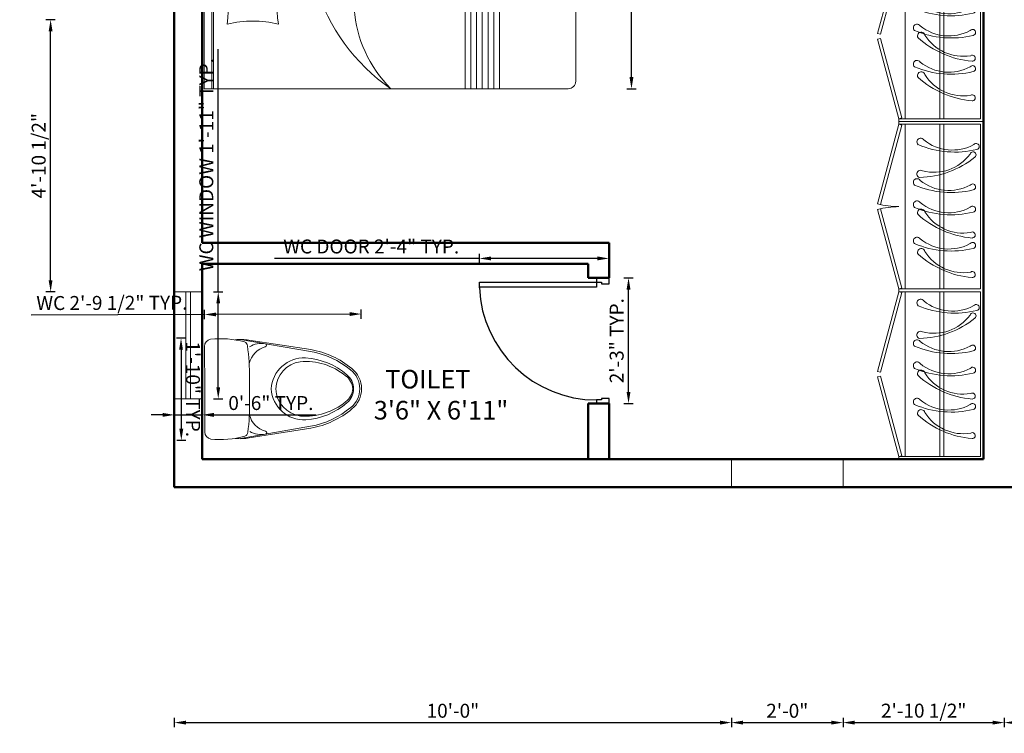
# Model space of a CAD drawing. Units: inches. Extents: x 1961 to 3038, y 800 to 1438.
# Tile 1 of 13: x 2592 to 2803, y 800 to 953. Entities that reach past the tile are written whole.
import ezdxf

# ---------------------------------------------------------------- set-up
doc = ezdxf.new("R2010")
doc.units = ezdxf.units.IN
for name, color, linetype, lineweight in [('A-ANNO-DIMS', 2, 'Continuous', 18), ('A-AREA-IDEN', 7, 'Continuous', 25), ('A-DOOR', 3, 'Continuous', 25), ('A-FLOR-FIXT', 9, 'Continuous', 18), ('A-FURN', 8, 'Continuous', 18), ('A-GLAZ', 4, 'Continuous', 18), ('A-WALL', 7, 'Continuous', 50)]:
    doc.layers.add(name, color=color, linetype=linetype, lineweight=lineweight)
doc.styles.get("Standard").update_dxf_attribs({"font": 'arial.ttf'})
doc.dimstyles.new('ISO-25', dxfattribs={"dimtxt": 3, "dimasz": 2.5, "dimexe": 1, "dimexo": 1, "dimtad": 1, "dimdec": 4, "dimlunit": 4, "dimtxsty": 'Standard', "dimcen": 2.5, "dimadec": 0, "dimazin": 0, "dimtfac": 1, "dimtdec": 4, "dimtmove": 0, "dimatfit": 3, "dimfxl": 1, "dimfxlon": 1, "dimarcsym": 0})

# ---------------------------------------------------------------- blocks, each defined once
blk = doc.blocks.new('door 23')
for p, q in [((2995, 1217.93), (2996.24, 1217.93)), ((2995.15, 1192.78), (2995.15, 1217.93)), ((2996.24, 1217.93), (2996.24, 1192.78)), ((2997.17, 1192.78), (2995.15, 1192.78)), ((2996.24, 1192.78), (2996.24, 1191.69)), ((2996.24, 1191.69), (2995.91, 1191.69)), ((2995.91, 1191.69), (2995.91, 1190.05)), ((2995.91, 1190.05), (2997.17, 1190.05))]:
    blk.add_line(p, q)
blk.add_lwpolyline([(2970.17, 1190.05), (2971.26, 1190.05), (2971.26, 1191.69), (2970.93, 1191.69), (2970.93, 1192.78), (2970.17, 1192.78)])
blk.add_arc((2996.1, 1192.78), 25.17, 92.4896, 180)
blk = doc.blocks.new('A$C41DA168A')
for p, q in [((151.4, 2380), (0, 1814.9)), ((151.4, 2380), (151.4, 2400)), ((151.4, 2400), (751.4, 2400)), ((731.4, 2380), (151.4, 2380)), ((170.7, 2374.8), (151.4, 2380)), ((196.6, 1210), (196.6, 2380)), ((441.4, 1210), (441.4, 2380)), ((471.4, 1210), (471.4, 2380)), ((731.4, 1210), (731.4, 2380)), ((751.4, 2400), (751.4, 0)), ((19.3, 1809.8), (170.7, 2374.8)), ((0, 1814.9), (19.3, 1809.8)), ((0, 1775.1), (19.3, 1780.2)), ((151.4, 1210), (0, 1775.1)), ((19.3, 1780.2), (170.7, 1215.2)), ((151.4, 1190), (0, 624.9)), ((170.7, 1215.2), (151.4, 1210)), ((151.4, 1210), (731.4, 1210)), ((151.4, 1190), (151.4, 1210)), ((731.4, 1190), (151.4, 1190)), ((170.7, 1184.8), (151.4, 1190)), ((196.6, 20), (196.6, 1190)), ((441.4, 1190), (441.4, 20)), ((471.4, 1190), (471.4, 20)), ((731.4, 20), (731.4, 1190)), ((19.3, 619.8), (170.7, 1184.8)), ((0, 624.9), (19.3, 619.8)), ((0, 585.1), (19.3, 590.2)), ((151.4, 20), (0, 585.1)), ((19.3, 590.2), (170.7, 25.2)), ((170.7, 25.2), (151.4, 20)), ((151.4, 0), (151.4, 20)), ((151.4, 20), (731.4, 20)), ((751.4, 0), (151.4, 0))]:
    blk.add_line(p, q)
for centre, radius, start, end in [((305.7, 2255.1), 26.3, 32.27517, 228.96506), ((530.9, 2518.7), 321.7, 230.8748, 298.39865), ((700.5, 2222.3), 21.4, 283.29422, 141.17028), ((548.2, 2849.7), 667, 247.08357, 283.63935), ((677.9, 2162.6), 21.4, 307.99916, 165.87521), ((277.3, 2668.9), 667, 271.7885, 308.34429), ((399.9, 2361), 321.7, 255.57974, 323.10358), ((305.5, 2027.4), 26.3, 56.9801, 253.67), ((280.2, 1967.6), 26.3, 32.27517, 228.96506), ((505.3, 2231.2), 321.7, 230.8748, 298.39865), ((522.6, 2562.2), 667, 247.08357, 283.63935), ((675, 1934.8), 21.4, 283.29422, 141.17028), ((280.2, 1809.7), 26.3, 32.27517, 228.96506), ((505.3, 2073.2), 321.7, 230.8748, 298.39865), ((151.4, 2380), 585, 255, 270), ((151.4, 1210), 585, 90, 105), ((522.6, 2404.2), 667, 247.08357, 283.63935), ((309.6, 1752), 26.3, 13.45499, 210.14489), ((607.8, 1928.8), 321.7, 212.05463, 279.57847), ((675, 1776.9), 21.4, 283.29422, 141.17028), ((730.9, 2236.5), 667, 228.26339, 264.81917), ((672.7, 1593.6), 21.4, 264.47404, 122.3501), ((280.2, 1552.2), 26.3, 32.27517, 228.96506), ((505.3, 1815.7), 321.7, 230.8748, 298.39865), ((675, 1519.4), 21.4, 283.29422, 141.17028), ((522.6, 2146.7), 667, 247.08357, 283.63935), ((309.6, 1470.8), 26.3, 13.45499, 210.14489), ((607.8, 1647.6), 321.7, 212.05463, 279.57847), ((730.9, 1955.3), 667, 228.26339, 264.81917), ((672.7, 1312.3), 21.4, 264.47404, 122.3501), ((305.7, 1111), 26.3, 32.27517, 228.96506), ((530.9, 1374.6), 321.7, 230.8748, 298.39865), ((548.2, 1705.5), 667, 247.08357, 283.63935), ((700.5, 1078.2), 21.4, 283.29422, 141.17028), ((277.3, 1524.8), 667, 271.7885, 308.34429), ((399.9, 1216.9), 321.7, 255.57974, 323.10358), ((677.9, 1018.5), 21.4, 307.99916, 165.87521), ((280.2, 823.5), 26.3, 32.27517, 228.96506), ((305.5, 883.3), 26.3, 56.9801, 253.67), ((522.6, 1418), 667, 247.08357, 283.63935), ((505.3, 1087.1), 321.7, 230.8748, 298.39865), ((675, 790.7), 21.4, 283.29422, 141.17028), ((280.2, 665.6), 26.3, 32.27517, 228.96506), ((522.6, 1260.1), 667, 247.08357, 283.63935), ((309.6, 607.9), 26.3, 13.45499, 210.14489), ((505.3, 929.1), 321.7, 230.8748, 298.39865), ((675, 632.8), 21.4, 283.29422, 141.17028), ((730.9, 1092.4), 667, 228.26339, 264.81917), ((607.8, 784.7), 321.7, 212.05463, 279.57847), ((280.2, 408.1), 26.3, 32.27517, 228.96506), ((505.3, 671.6), 321.7, 230.8748, 298.39865), ((672.7, 449.5), 21.4, 264.47404, 122.3501), ((522.6, 1002.6), 667, 247.08357, 283.63935), ((309.6, 326.7), 26.3, 13.45499, 210.14489), ((675, 375.3), 21.4, 283.29422, 141.17028), ((730.9, 811.2), 667, 228.26339, 264.81917), ((607.8, 503.5), 321.7, 212.05463, 279.57847), ((672.7, 168.2), 21.4, 264.47404, 122.3501)]:
    blk.add_arc(centre, radius, start, end)
blk = doc.blocks.new('A$C11850ECD')
for p, q in [((0, 1.95), (0, 0.04)), ((0, 1.95), (1.2, 1.95)), ((1.2, 1.95), (1.2, 0.04)), ((1.2318, 1.952), (1.8168, 1.952)), ((1.2318, 1.367), (1.2318, 1.952)), ((1.5243, 1.952), (1.5243, 1.7225)), ((1.8168, 1.952), (1.8168, 1.367)), ((0, 1.91), (1.2, 1.91)), ((0, 1.9), (1.2, 1.9)), ((1.4613, 1.6586), (1.2318, 1.6586)), ((1.8168, 1.6595), (1.5873, 1.6595)), ((1.5243, 1.5965), (1.5243, 1.367)), ((1.8168, 1.367), (1.2318, 1.367)), ((0, 0.58), (1.2, 0.58)), ((0, 0.55), (1.2, 0.55)), ((0, 0.52), (1.2, 0.52)), ((0, 0.49), (1.2, 0.49)), ((0, 0.46), (1.2, 0.46)), ((0, 0.43), (1.2, 0.43)), ((0, 0.4), (1.2, 0.4)), ((1.16, 0), (0.04, 0))]:
    blk.add_line(p, q)
for radius in [0.27, 0.09]:
    blk.add_circle((1.5243, 1.6595), radius)
for centre, radius, start, end in [((-0.2053, 1.694), 0.5605, 346.15, 13.85), ((0.5998, 5.1077), 3.2899, 265.4501, 274.5499), ((0.3425, 1.5416), 0.3789, 4.7708, 46.8165), ((0.3425, 1.5416), 0.4089, 4.1373, 42.5614), ((0.3425, 1.5416), 0.4389, 3.5318, 39.1874), ((0.3425, 1.5416), 0.4689, 2.9489, 36.4321), ((1.3429, 1.694), 0.5004, 164.4468, 195.5532), ((0.5998, -0.4629), 2.0395, 82.6483, 97.3517), ((0.8389, 0.3894), 1.0202, 69.2731, 145.3133), ((1.3044, 0.8859), 0.4695, 102.8515, 161.769), ((0.4655, 0.5058), 0.6574, 53.2823, 135.0802), ((0.04, 0.04), 0.04, 180, 270), ((1.16, 0.04), 0.04, 270, 0)]:
    blk.add_arc(centre, radius, start, end)
blk = doc.blocks.new('A$C188A4A68')
at = {"ltscale": 20}
for p, q in [((0.2444, 0.7693), (0.0344, 0.7693)), ((0.2444, 0.7693), (0.4544, 0.7693)), ((0.0013, 0.5938), (0.0607, 0.2504)), ((0.4874, 0.5938), (0.428, 0.2504)), ((0.0054, 0.5515), (0.0519, 0.2489)), ((0.2444, 0.5498), (0.1889, 0.5498)), ((0.2444, 0.5498), (0.2998, 0.5498)), ((0.4833, 0.5515), (0.4368, 0.2489))]:
    blk.add_line(p, q, dxfattribs=at)
for centre, radius, start, end in [((0.442, 0.6914), 0.4447, 173.6395, 195.464), ((0.0344, 0.7343), 0.0349, 90, 169.5926), ((0.4544, 0.7343), 0.0349, 10.4074, 90), ((0.0467, 0.6914), 0.4447, 344.536, 6.3605), ((0.2125, 0.5932), 0.2113, 172.6498, 191.3659), ((0.2762, 0.5932), 0.2113, 348.6341, 7.3502), ((0.0333, 0.5802), 0.0213, 200.243, 267.1503), ((0.1303, 0.4913), 0.1097, 148.5069, 190.0488), ((0.1632, 1.4554), 0.906, 261.6902, 271.6258), ((0.1461, 0.4405), 0.1134, 104.1041, 164.1501), ((0.3255, 1.4554), 0.906, 268.3742, 278.3098), ((0.3426, 0.4405), 0.1134, 15.8499, 75.8959), ((0.3584, 0.4913), 0.1097, 349.9512, 31.4931), ((0.4554, 0.5802), 0.0213, 272.8497, 339.757), ((0.0297, 0.4734), 0.0075, 189.8264, 345.0875), ((0.254, 0.2824), 0.1613, 93.4333, 183.0038), ((0.2347, 0.2824), 0.1613, 356.9962, 86.5667), ((0.459, 0.4734), 0.0075, 194.9125, 350.1736), ((0.2493, 0.2813), 0.1393, 92.0329, 172.0373), ((0.2394, 0.2813), 0.1393, 7.9627, 87.9671), ((0.4211, 0.2752), 0.3108, 175.3213, 219.2477), ((0.0676, 0.2752), 0.3108, 320.7523, 4.6787), ((0.4781, 0.3243), 0.4328, 190.0297, 219.7428), ((0.4781, 0.3243), 0.4238, 190.0435, 219.7538), ((0.4311, 0.2946), 0.3389, 183.5042, 221.0229), ((0.0576, 0.2946), 0.3389, 318.9771, 356.4958), ((0.0106, 0.3243), 0.4238, 320.2462, 349.9565), ((0.0106, 0.3243), 0.4328, 320.2572, 349.9703), ((0.2444, 0.127), 0.118, 218.6774, 270), ((0.2444, 0.127), 0.088, 218.504, 270), ((0.2498, 0.1282), 0.0854, 215.5685, 266.3197), ((0.2389, 0.1282), 0.0854, 273.6803, 324.4315), ((0.2444, 0.127), 0.088, 270, 321.496), ((0.2444, 0.127), 0.118, 270, 321.3226), ((0.2444, 0.127), 0.127, 218.716, 270), ((0.2444, 0.127), 0.127, 270, 321.284)]:
    blk.add_arc(centre, radius, start, end, dxfattribs=at)
blk = doc.blocks.new('WIN-23IN')
for p, q in [((0, 23), (6, 23)), ((2.5, 23), (2.5, 0)), ((3.5, 23), (3.5, 0)), ((0, 0), (6, 0))]:
    blk.add_line(p, q)
blk = doc.blocks.new('*D35')
at = {"layer": 'A-ANNO-DIMS', "color": 0, "lineweight": -2, "transparency": 16777216}
for p, q in [((2690.39, 902.1), (2646.35, 902.1)), ((2690.39, 901.1), (2690.39, 903.1)), ((2715.77, 902.1), (2692.89, 902.1)), ((2718.27, 901.1), (2718.27, 903.1))]:
    blk.add_line(p, q, dxfattribs=at)
at = {"layer": 'A-ANNO-DIMS', "color": 0, "transparency": 16777216}
for points in [[(2692.89, 902.52), (2692.89, 901.68), (2690.39, 902.1)], [(2715.77, 902.52), (2715.77, 901.68), (2718.27, 902.1)]]:
    blk.add_solid(points, dxfattribs=at)
at = {"layer": 'Defpoints', "color": 0, "transparency": 16777216}
for p in [(2690.39, 902.1), (2690.39, 897.92), (2718.27, 897.92)]:
    blk.add_point(p, dxfattribs=at)
at = {"layer": 'A-ANNO-DIMS', "color": 0, "transparency": 16777216, "insert": (2667.12, 904.28), "char_height": 3, "attachment_point": 5}
blk.add_mtext('WC DOOR 2\'-4" TYP.', dxfattribs=at)
blk = doc.blocks.new('*D36')
at = {"layer": 'A-ANNO-DIMS', "color": 0, "lineweight": -2, "transparency": 16777216}
for p, q in [((2721.45, 897.92), (2723.45, 897.92)), ((2722.45, 873.42), (2722.45, 895.42)), ((2721.45, 870.92), (2723.45, 870.92))]:
    blk.add_line(p, q, dxfattribs=at)
at = {"layer": 'A-ANNO-DIMS', "color": 0, "transparency": 16777216}
for points in [[(2722.03, 895.42), (2722.87, 895.42), (2722.45, 897.92)], [(2722.03, 873.42), (2722.87, 873.42), (2722.45, 870.92)]]:
    blk.add_solid(points, dxfattribs=at)
at = {"layer": 'Defpoints', "color": 0, "transparency": 16777216}
for p in [(2718.27, 897.92), (2722.45, 897.92), (2718.27, 870.92)]:
    blk.add_point(p, dxfattribs=at)
at = {"layer": 'A-ANNO-DIMS', "color": 0, "transparency": 16777216, "insert": (2720.29, 884.42), "char_height": 3, "attachment_point": 5, "rotation": 90}
blk.add_mtext('2\'-3" TYP.', dxfattribs=at)
blk = doc.blocks.new('*D41')
at = {"layer": 'A-ANNO-DIMS', "color": 0, "lineweight": -2, "transparency": 16777216}
for p, q in [((2631.25, 890.05), (2593.96, 889.93)), ((2631.26, 889.05), (2631.25, 891.05)), ((2662.49, 890.14), (2633.75, 890.05)), ((2664.99, 889.15), (2664.99, 891.15))]:
    blk.add_line(p, q, dxfattribs=at)
at = {"layer": 'A-ANNO-DIMS', "color": 0, "transparency": 16777216}
for points in [[(2633.75, 890.47), (2633.76, 889.64), (2631.25, 890.05)], [(2662.49, 890.56), (2662.49, 889.73), (2664.99, 890.15)]]:
    blk.add_solid(points, dxfattribs=at)
at = {"layer": 'Defpoints', "color": 0, "transparency": 16777216}
for p in [(2631.25, 890.05), (2631.27, 884.99), (2665.01, 885.09)]:
    blk.add_point(p, dxfattribs=at)
at = {"layer": 'A-ANNO-DIMS', "color": 0, "transparency": 16777216, "insert": (2611.35, 892.16), "char_height": 3, "attachment_point": 5, "rotation": 0.1765}
blk.add_mtext('WC 2\'-9 1/2" TYP.', dxfattribs=at)
blk = doc.blocks.new('*D42')
at = {"layer": 'A-ANNO-DIMS', "color": 0, "lineweight": -2, "transparency": 16777216}
for p, q in [((2627.21, 884.97), (2625.21, 884.97)), ((2626.22, 882.47), (2626.27, 865.49)), ((2627.28, 862.99), (2625.28, 862.99))]:
    blk.add_line(p, q, dxfattribs=at)
at = {"layer": 'A-ANNO-DIMS', "color": 0, "transparency": 16777216}
for points in [[(2626.63, 882.47), (2625.8, 882.47), (2626.21, 884.97)], [(2626.69, 865.49), (2625.85, 865.49), (2626.28, 862.99)]]:
    blk.add_solid(points, dxfattribs=at)
at = {"layer": 'Defpoints', "color": 0, "transparency": 16777216}
for p in [(2631.27, 884.99), (2626.28, 862.99), (2631.34, 863)]:
    blk.add_point(p, dxfattribs=at)
at = {"layer": 'A-ANNO-DIMS', "color": 0, "transparency": 16777216, "insert": (2628.4, 873.99), "char_height": 3, "attachment_point": 5, "rotation": 270.1765}
blk.add_mtext('1\'-10" TYP.', dxfattribs=at)
blk = doc.blocks.new('*D43')
at = {"layer": 'A-ANNO-DIMS', "color": 0, "lineweight": -2, "transparency": 16777216}
for p, q in [((2634.22, 894.92), (2634.22, 947.11)), ((2633.22, 894.92), (2635.22, 894.92)), ((2634.22, 874.42), (2634.22, 892.42)), ((2633.22, 871.92), (2635.22, 871.92))]:
    blk.add_line(p, q, dxfattribs=at)
at = {"layer": 'A-ANNO-DIMS', "color": 0, "transparency": 16777216}
for points in [[(2633.8, 892.42), (2634.63, 892.42), (2634.22, 894.92)], [(2633.8, 874.42), (2634.63, 874.42), (2634.22, 871.92)]]:
    blk.add_solid(points, dxfattribs=at)
at = {"layer": 'Defpoints', "color": 0, "transparency": 16777216}
for p in [(2630.77, 894.92), (2634.22, 894.92), (2630.77, 871.92)]:
    blk.add_point(p, dxfattribs=at)
at = {"layer": 'A-ANNO-DIMS', "color": 0, "transparency": 16777216, "insert": (2632.04, 922.26), "char_height": 3, "attachment_point": 5, "rotation": 90}
blk.add_mtext('WC WINDOW 1\'-11" TYP.', dxfattribs=at)
blk = doc.blocks.new('*D44')
at = {"layer": 'A-ANNO-DIMS', "color": 0, "lineweight": -2, "transparency": 16777216}
for p, q in [((2622.27, 868.47), (2619.77, 868.47)), ((2624.77, 869.47), (2624.77, 867.47)), ((2624.77, 868.47), (2630.77, 868.47)), ((2630.77, 869.47), (2630.77, 867.47)), ((2633.27, 868.47), (2655.3, 868.47))]:
    blk.add_line(p, q, dxfattribs=at)
at = {"layer": 'A-ANNO-DIMS', "color": 0, "transparency": 16777216}
for points in [[(2622.27, 868.89), (2622.27, 868.05), (2624.77, 868.47)], [(2633.27, 868.89), (2633.27, 868.05), (2630.77, 868.47)]]:
    blk.add_solid(points, dxfattribs=at)
at = {"layer": 'Defpoints', "color": 0, "transparency": 16777216}
for p in [(2624.77, 871.92), (2630.77, 871.92), (2630.77, 868.47)]:
    blk.add_point(p, dxfattribs=at)
at = {"layer": 'A-ANNO-DIMS', "color": 0, "transparency": 16777216, "insert": (2645.54, 870.63), "char_height": 3, "attachment_point": 5}
blk.add_mtext('0\'-6" TYP.', dxfattribs=at)
blk = doc.blocks.new('*D58')
at = {"layer": 'A-ANNO-DIMS', "color": 0, "lineweight": -2, "transparency": 16777216}
for p, q in [((2722.09, 1013.03), (2724.09, 1013.03)), ((2723.09, 941.07), (2723.09, 1010.53)), ((2722.09, 938.57), (2724.09, 938.57))]:
    blk.add_line(p, q, dxfattribs=at)
at = {"layer": 'A-ANNO-DIMS', "color": 0, "transparency": 16777216}
for points in [[(2722.67, 1010.53), (2723.5, 1010.53), (2723.09, 1013.03)], [(2722.67, 941.07), (2723.5, 941.07), (2723.09, 938.57)]]:
    blk.add_solid(points, dxfattribs=at)
at = {"layer": 'Defpoints', "color": 0, "transparency": 16777216}
for p in [(2711.09, 1013.03), (2723.09, 1013.03), (2711.09, 938.57)]:
    blk.add_point(p, dxfattribs=at)
at = {"layer": 'A-ANNO-DIMS', "color": 0, "transparency": 16777216, "insert": (2720.91, 975.8), "char_height": 3, "attachment_point": 5, "rotation": 90}
blk.add_mtext('6\'-2 1/2"', dxfattribs=at)
blk = doc.blocks.new('*D71')
at = {"layer": 'A-ANNO-DIMS', "color": 0, "lineweight": -2, "transparency": 16777216}
for p, q in [((2803.27, 803.32), (2803.27, 801.32)), ((2851.27, 803.32), (2851.27, 801.32)), ((2805.77, 802.32), (2848.77, 802.32))]:
    blk.add_line(p, q, dxfattribs=at)
at = {"layer": 'A-ANNO-DIMS', "color": 0, "transparency": 16777216}
for points in [[(2805.77, 802.74), (2805.77, 801.9), (2803.27, 802.32)], [(2848.77, 802.74), (2848.77, 801.9), (2851.27, 802.32)]]:
    blk.add_solid(points, dxfattribs=at)
at = {"layer": 'Defpoints', "color": 0, "transparency": 16777216}
for p in [(2803.27, 828.92), (2851.27, 828.92), (2851.27, 802.32)]:
    blk.add_point(p, dxfattribs=at)
at = {"layer": 'A-ANNO-DIMS', "color": 0, "transparency": 16777216, "insert": (2827.27, 804.48), "char_height": 3, "attachment_point": 5}
blk.add_mtext('4\'-0"', dxfattribs=at)
blk = doc.blocks.new('*D74')
at = {"layer": 'A-ANNO-DIMS', "color": 0, "lineweight": -2, "transparency": 16777216}
for p, q in [((2744.59, 803.32), (2744.59, 801.32)), ((2768.59, 803.32), (2768.59, 801.32)), ((2747.09, 802.32), (2766.09, 802.32))]:
    blk.add_line(p, q, dxfattribs=at)
at = {"layer": 'A-ANNO-DIMS', "color": 0, "transparency": 16777216}
for points in [[(2747.09, 802.74), (2747.09, 801.9), (2744.59, 802.32)], [(2766.09, 802.74), (2766.09, 801.9), (2768.59, 802.32)]]:
    blk.add_solid(points, dxfattribs=at)
at = {"layer": 'Defpoints', "color": 0, "transparency": 16777216}
for p in [(2744.59, 852.92), (2768.59, 852.92), (2768.59, 802.32)]:
    blk.add_point(p, dxfattribs=at)
at = {"layer": 'A-ANNO-DIMS', "color": 0, "transparency": 16777216, "insert": (2756.59, 804.48), "char_height": 3, "attachment_point": 5}
blk.add_mtext('2\'-0"', dxfattribs=at)
blk = doc.blocks.new('*D82')
at = {"layer": 'A-ANNO-DIMS', "color": 0, "lineweight": -2, "transparency": 16777216}
for p, q in [((2599.17, 953.42), (2597.17, 953.42)), ((2598.17, 897.42), (2598.17, 950.92)), ((2599.17, 894.92), (2597.17, 894.92))]:
    blk.add_line(p, q, dxfattribs=at)
at = {"layer": 'A-ANNO-DIMS', "color": 0, "transparency": 16777216}
for points in [[(2597.75, 950.92), (2598.58, 950.92), (2598.17, 953.42)], [(2597.75, 897.42), (2598.58, 897.42), (2598.17, 894.92)]]:
    blk.add_solid(points, dxfattribs=at)
at = {"layer": 'Defpoints', "color": 0, "transparency": 16777216}
for p in [(2598.17, 953.42), (2624.77, 953.42), (2624.77, 894.92)]:
    blk.add_point(p, dxfattribs=at)
at = {"layer": 'A-ANNO-DIMS', "color": 0, "transparency": 16777216, "insert": (2595.99, 924.17), "char_height": 3, "attachment_point": 5, "rotation": 90}
blk.add_mtext('4\'-10 1/2"', dxfattribs=at)
blk = doc.blocks.new('*D84')
at = {"layer": 'A-ANNO-DIMS', "color": 0, "lineweight": -2, "transparency": 16777216}
for p, q in [((2624.77, 803.32), (2624.77, 801.32)), ((2744.59, 803.32), (2744.59, 801.32)), ((2627.27, 802.32), (2742.09, 802.32))]:
    blk.add_line(p, q, dxfattribs=at)
at = {"layer": 'A-ANNO-DIMS', "color": 0, "transparency": 16777216}
for points in [[(2627.27, 802.74), (2627.27, 801.9), (2624.77, 802.32)], [(2742.09, 802.74), (2742.09, 801.9), (2744.59, 802.32)]]:
    blk.add_solid(points, dxfattribs=at)
at = {"layer": 'Defpoints', "color": 0, "transparency": 16777216}
for p in [(2624.77, 852.92), (2744.59, 852.92), (2744.59, 802.32)]:
    blk.add_point(p, dxfattribs=at)
at = {"layer": 'A-ANNO-DIMS', "color": 0, "transparency": 16777216, "insert": (2684.68, 804.48), "char_height": 3, "attachment_point": 5}
blk.add_mtext('10\'-0"', dxfattribs=at)
blk = doc.blocks.new('*D85')
at = {"layer": 'A-ANNO-DIMS', "color": 0, "lineweight": -2, "transparency": 16777216}
for p, q in [((2768.59, 803.32), (2768.59, 801.32)), ((2803.27, 803.32), (2803.27, 801.32)), ((2771.09, 802.32), (2800.77, 802.32))]:
    blk.add_line(p, q, dxfattribs=at)
at = {"layer": 'A-ANNO-DIMS', "color": 0, "transparency": 16777216}
for points in [[(2771.09, 802.74), (2771.09, 801.9), (2768.59, 802.32)], [(2800.77, 802.74), (2800.77, 801.9), (2803.27, 802.32)]]:
    blk.add_solid(points, dxfattribs=at)
at = {"layer": 'Defpoints', "color": 0, "transparency": 16777216}
for p in [(2768.59, 852.92), (2803.27, 828.92), (2803.27, 802.32)]:
    blk.add_point(p, dxfattribs=at)
at = {"layer": 'A-ANNO-DIMS', "color": 0, "transparency": 16777216, "insert": (2785.93, 804.5), "char_height": 3, "attachment_point": 5}
blk.add_mtext('2\'-10 1/2"', dxfattribs=at)

msp = doc.modelspace()

# ---------------------------------------------------------------- linework, layer by layer
at = {"layer": 'A-GLAZ'}
for p, q in [((2744.59389, 858.91975), (2744.59389, 852.91975)), ((2768.59389, 858.91975), (2768.59389, 852.91975))]:
    msp.add_line(p, q, dxfattribs=at)
at = {"layer": 'A-WALL'}
for p, q in [((2624.76803, 1314.91975), (2624.76803, 852.91975)), ((2630.76803, 1053.91975), (2630.76803, 905.41975)), ((2798.76803, 1053.91975), (2798.76803, 858.91975)), ((2630.76803, 905.41975), (2718.26803, 905.41975)), ((2718.26803, 905.41975), (2718.26803, 897.91975)), ((2630.76803, 900.91975), (2713.76803, 900.91975)), ((2630.76803, 900.91975), (2630.76803, 858.91975)), ((2713.76803, 900.91975), (2713.76803, 897.91975)), ((2713.76803, 897.91975), (2718.26803, 897.91975)), ((2713.76803, 870.91975), (2718.26803, 870.91975)), ((2713.76803, 870.91975), (2713.76803, 858.91975)), ((2718.26803, 870.91975), (2718.26803, 858.91975)), ((2630.76803, 858.91975), (2798.76803, 858.91975)), ((2624.76803, 852.91975), (3008.76803, 852.91975))]:
    msp.add_line(p, q, dxfattribs=at)

# ---------------------------------------------------------------- block references
at = {"layer": 'A-DOOR', "rotation": 90.00000000000003}
msp.add_blockref('door 23', (3908.31489, -2099.24731), dxfattribs=at)
at = {"layer": 'A-FLOR-FIXT', "xscale": -43.8549224568521, "yscale": 43.8549224568521, "zscale": 43.8549224568521, "rotation": 90.17652575876701}
msp.add_blockref('A$C188A4A68', (2665.00618, 884.815), dxfattribs=at)
at = {"layer": 'A-FURN', "xscale": 40.98381615062051, "yscale": 40.98381615062051, "zscale": 40.98381615062051, "rotation": 90}
msp.add_blockref('A$C11850ECD', (2711.08548, 938.57032), dxfattribs=at)
at = {"layer": 'A-FURN', "xscale": 0.0302586277246643, "yscale": 0.0302586277246643, "zscale": 0.0302586277246643}
for p in [(2776.03142, 931.54046), (2776.03142, 858.91975)]:
    msp.add_blockref('A$C41DA168A', p, dxfattribs=at)
at = {"layer": 'A-GLAZ'}
msp.add_blockref('WIN-23IN', (2624.768, 871.92), dxfattribs=at)

# ---------------------------------------------------------------- texts
at = {"layer": 'A-AREA-IDEN', "insert": (2667.66577, 878.14249), "char_height": 4, "attachment_point": 1}
msp.add_mtext_dynamic_manual_height_columns('{\\fTimes New Roman|b1|i0|c0|p18;  TOILET\\P3\'6" X 6\'11"}', width=33.1080891, gutter_width=12.5, heights=[0], dxfattribs=at)

# ---------------------------------------------------------------- dimensions: what is measured, and where the dimension line sits
at = {"layer": 'A-ANNO-DIMS'}
for base, p1, p2, picture, middle in [((2723.08548, 1013.02777), (2711.08548, 938.57031), (2711.08548, 1013.02777), '*D58', (2720.90932, 975.79904)), ((2598.16803, 953.41975), (2624.76803, 894.91975), (2624.76803, 953.41975), '*D82', (2595.99187, 924.16975))]:
    dim = msp.add_linear_dim(base=base, p1=p1, p2=p2, angle=90, dimstyle='ISO-25', override={"dimdec": 1, "dimlfac": 1, "dimrnd": 0, "dimzin": 1, "dimdsep": 46, "dimlunit": 4, "dimfrac": 2}, dxfattribs=at)
    dim.commit()
    dim.dimension.update_dxf_attribs({"geometry": picture, "text_midpoint": middle})
for base, p1, p2, angle, text, picture, middle in [((2634.21803, 894.91975), (2630.76803, 871.91975), (2630.76803, 894.91975), 90, 'WC WINDOW <> TYP.', '*D43', (2632.04085, 922.26474)), ((2690.38896, 902.10161), (2718.26803, 897.91975), (2690.38896, 897.91975), 180, 'WC DOOR <> TYP.', '*D35', (2667.11731, 904.2788)), ((2631.25431, 890.04654), (2665.00533, 885.09016), (2631.2699, 884.98622), 180.1765258, 'WC <> TYP.', '*D41', (2611.34951, 892.16138)), ((2722.44989, 897.91975), (2718.26803, 870.91975), (2718.26803, 897.91975), 90, '<> TYP.', '*D36', (2720.29215, 884.41975)), ((2626.27732, 862.98848), (2631.2699, 884.98622), (2631.33763, 863.00407), 270.1765258, '<> TYP.', '*D42', (2628.40016, 873.9862))]:
    dim = msp.add_linear_dim(base=base, p1=p1, p2=p2, angle=angle, text=text, dimstyle='ISO-25', override={"dimdec": 1, "dimlfac": 1, "dimrnd": 0, "dimzin": 1, "dimdsep": 46, "dimlunit": 4, "dimfrac": 2}, dxfattribs=at)
    dim.commit()
    dim.dimension.update_dxf_attribs({"geometry": picture, "text_midpoint": middle})
dim = msp.add_linear_dim(base=(2630.76803, 868.46975), p1=(2624.76803, 871.91975), p2=(2630.76803, 871.91975), text='<> TYP.', dimstyle='ISO-25', override={"dimdec": 1, "dimlfac": 1, "dimrnd": 0, "dimzin": 1, "dimdsep": 46, "dimlunit": 4, "dimfrac": 2}, dxfattribs=at)
dim.commit()
dim.dimension.update_dxf_attribs({"geometry": '*D44', "text_midpoint": (2645.53628, 870.62647)})
for base, p1, p2, picture, middle in [((2744.59389, 802.31975), (2624.76803, 852.91975), (2744.59389, 852.91975), '*D84', (2684.68096, 804.47647)), ((2768.59389, 802.31975), (2744.59389, 852.91975), (2768.59389, 852.91975), '*D74', (2756.59389, 804.47647)), ((2803.26803, 802.31975), (2768.59389, 852.91975), (2803.26803, 828.91975), '*D85', (2785.93096, 804.49591)), ((2851.26803, 802.31975), (2803.26803, 828.91975), (2851.26803, 828.91975), '*D71', (2827.26803, 804.47647))]:
    dim = msp.add_linear_dim(base=base, p1=p1, p2=p2, dimstyle='ISO-25', override={"dimdec": 1, "dimlfac": 1, "dimrnd": 0, "dimzin": 1, "dimdsep": 46, "dimlunit": 4, "dimfrac": 2}, dxfattribs=at)
    dim.commit()
    dim.dimension.update_dxf_attribs({"geometry": picture, "text_midpoint": middle})

doc.saveas('drawing.dxf')
